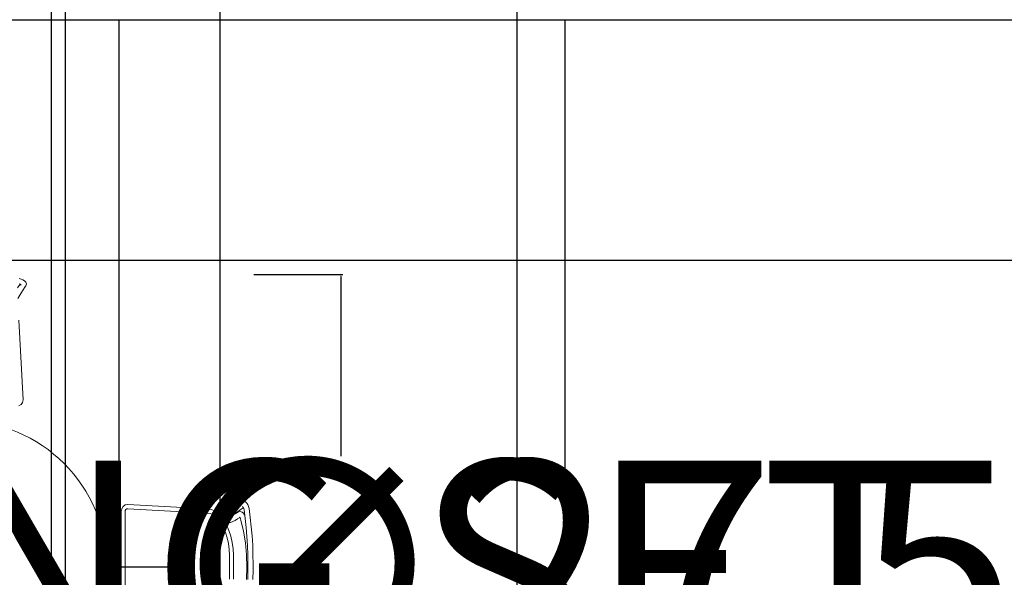
# Model space of a CAD drawing. Units: inches. Extents: x 305 to 776, y 38 to 479.
# Tile 11 of 14: x 419 to 511, y 280 to 332. Entities that reach past the tile are written whole.
import ezdxf

# ---------------------------------------------------------------- set-up
doc = ezdxf.new("R2010")
doc.units = ezdxf.units.IN
doc.header["$MEASUREMENT"] = 0
doc.layers.add('A-ANNO-DIMS', color=2, linetype='Continuous', lineweight=18)
doc.layers.add('A-FURN', color=8, linetype='Continuous', lineweight=18)
doc.styles.get("Standard").update_dxf_attribs({"font": 'arial.ttf'})
doc.dimstyles.get("Standard").update_dxf_attribs({"dimtxt": 20, "dimasz": 0.18, "dimexe": 0.18, "dimexo": 0.0625, "dimgap": 0.09, "dimtad": 0, "dimtih": 1, "dimtoh": 1, "dimdec": 4, "dimzin": 0, "dimdsep": 46, "dimtxsty": 'Standard', "dimcen": 0.09, "dimadec": 0, "dimazin": 0, "dimtfac": 1, "dimtdec": 4, "dimtofl": 0, "dimtmove": 0, "dimatfit": 3, "dimfxl": 1, "dimtolj": 1, "dimtzin": 0, "dimarcsym": 0})

# ---------------------------------------------------------------- blocks, each defined once
blk = doc.blocks.new('D')
for p, q in [((1089.75, 532.53), (1089.48, 532.6)), ((1089.75, 532.53), (1089.48, 532.6)), ((1089.62, 531.85), (1089.49, 531.9)), ((1089.97, 532.44), (1089.75, 532.53)), ((1089.97, 532.44), (1089.75, 532.53)), ((1090.18, 532.32), (1089.97, 532.44)), ((1090.18, 532.32), (1089.97, 532.44)), ((1090.35, 532.14), (1090.18, 532.32)), ((1090.35, 532.14), (1090.18, 532.32)), ((1090.39, 532.03), (1090.35, 532.14)), ((1090.35, 532.14), (1090.39, 532.03)), ((1090.43, 531.89), (1090.39, 532.03)), ((1090.43, 531.89), (1090.39, 532.03)), ((1090.4, 531.77), (1090.43, 531.89)), ((1090.43, 531.89), (1090.4, 531.77)), ((1089.27, 531.38), (1089.61, 531.85)), ((1089.58, 530.46), (1089.93, 531)), ((1089.58, 530.46), (1089.93, 531)), ((1089.69, 531.81), (1089.62, 531.85)), ((1089.78, 531.72), (1089.69, 531.81)), ((1089.93, 531), (1090.33, 531.61)), ((1089.93, 531), (1090.33, 531.61)), ((1090.33, 531.61), (1090.37, 531.66)), ((1090.37, 531.66), (1090.33, 531.61)), ((1090.37, 531.66), (1090.4, 531.77)), ((1090.37, 531.66), (1090.4, 531.77)), ((1089.31, 530.03), (1089.58, 530.46)), ((1089.31, 530.03), (1089.58, 530.46)), ((1090.02, 516.87), (1089.45, 527.19)), ((1090.02, 516.88), (1089.45, 527.19)), ((1089.95, 516.55), (1090.02, 516.88)), ((1089.95, 516.55), (1090.02, 516.87)), ((1089.44, 516.1), (1089.74, 516.28)), ((1089.44, 516.1), (1089.74, 516.28)), ((1089.74, 516.28), (1089.95, 516.55)), ((1089.74, 516.28), (1089.95, 516.55)), ((1102.72, 502.39), (1102.79, 502.75)), ((1102.72, 502.39), (1102.79, 502.75)), ((1102.79, 502.75), (1102.97, 503.06)), ((1102.79, 502.75), (1102.97, 503.06)), ((1102.97, 503.06), (1103.24, 503.26)), ((1102.97, 503.06), (1103.24, 503.26)), ((1103.24, 503.26), (1103.56, 503.33)), ((1103.24, 503.26), (1103.56, 503.33)), ((1103.33, 502.65), (1103.25, 502.53)), ((1103.43, 502.74), (1103.33, 502.65)), ((1103.56, 502.77), (1103.43, 502.74)), ((1103.56, 503.33), (1113.87, 502.77)), ((1103.56, 503.33), (1113.87, 502.77)), ((1113.85, 502.2), (1103.56, 502.77)), ((1113.87, 502.77), (1114.37, 502.68)), ((1113.87, 502.77), (1114.37, 502.68)), ((1114.37, 502.68), (1114.85, 502.5)), ((1114.37, 502.68), (1114.85, 502.5)), ((1116.01, 502.14), (1116.72, 502.62)), ((1116.01, 502.14), (1116.72, 502.62)), ((1116.72, 502.62), (1117.14, 502.89)), ((1116.72, 502.62), (1117.14, 502.89)), ((1117.14, 502.89), (1117.69, 503.24)), ((1117.14, 502.89), (1117.69, 503.24)), ((1117.56, 502.18), (1118.07, 502.58)), ((1117.69, 503.24), (1118.3, 503.64)), ((1117.69, 503.24), (1118.3, 503.64)), ((1118.07, 502.58), (1118.54, 502.93)), ((1118.3, 503.64), (1118.35, 503.68)), ((1118.35, 503.68), (1118.3, 503.64)), ((1118.35, 503.68), (1118.45, 503.71)), ((1118.35, 503.68), (1118.46, 503.71)), ((1118.41, 503.09), (1118.49, 503)), ((1118.45, 503.71), (1118.58, 503.74)), ((1118.58, 503.74), (1118.46, 503.71)), ((1118.49, 503), (1118.53, 502.93)), ((1118.53, 502.93), (1118.59, 502.8)), ((1118.58, 503.74), (1118.72, 503.7)), ((1118.58, 503.74), (1118.72, 503.7)), ((1118.59, 502.8), (1118.63, 502.63)), ((1118.63, 502.63), (1118.77, 501.51)), ((1118.72, 503.7), (1118.83, 503.66)), ((1118.83, 503.66), (1118.72, 503.7)), ((1118.83, 503.66), (1119.01, 503.49)), ((1118.83, 503.66), (1119.01, 503.49)), ((1119.01, 503.49), (1119.13, 503.29)), ((1119.01, 503.49), (1119.13, 503.29)), ((1119.13, 503.29), (1119.22, 503.06)), ((1119.13, 503.29), (1119.22, 503.06)), ((1119.22, 503.06), (1119.29, 502.79)), ((1119.22, 503.06), (1119.29, 502.79)), ((1119.29, 502.79), (1119.44, 501.61)), ((1119.29, 502.79), (1119.44, 501.61)), ((1102.72, 488.01), (1102.72, 502.39)), ((1102.72, 488.01), (1102.72, 502.39)), ((1103.25, 502.53), (1103.23, 502.39)), ((1103.23, 502.39), (1103.23, 488.01)), ((1114.27, 502.13), (1113.85, 502.2)), ((1114.68, 501.97), (1114.27, 502.13)), ((1115.05, 501.72), (1114.68, 501.97)), ((1114.85, 502.5), (1115.29, 502.22)), ((1114.85, 502.5), (1115.29, 502.22)), ((1115.37, 501.4), (1115.05, 501.72)), ((1115.29, 502.22), (1115.84, 501.82)), ((1115.29, 502.22), (1115.84, 501.82)), ((1115.63, 501.02), (1115.37, 501.4)), ((1115.84, 501.82), (1115.88, 501.74)), ((1116.37, 500.71), (1115.84, 501.82)), ((1115.88, 501.74), (1115.9, 501.76)), ((1115.89, 501.83), (1115.9, 501.9)), ((1115.9, 501.76), (1115.89, 501.83)), ((1115.9, 501.86), (1115.93, 502.01)), ((1115.9, 501.9), (1115.91, 501.96)), ((1115.91, 501.71), (1115.9, 501.86)), ((1115.91, 501.96), (1115.94, 502.03)), ((1115.98, 501.57), (1115.91, 501.71)), ((1115.93, 502.01), (1116.01, 502.14)), ((1115.94, 502.03), (1115.97, 502.09)), ((1115.97, 502.09), (1116.01, 502.14)), ((1116.08, 501.47), (1115.98, 501.57)), ((1116.21, 501.41), (1116.08, 501.47)), ((1116.35, 501.41), (1116.21, 501.41)), ((1116.48, 501.47), (1116.35, 501.41)), ((1116.66, 501.63), (1116.48, 501.47)), ((1116.53, 501.37), (1116.56, 501.49)), ((1116.54, 501.24), (1116.53, 501.37)), ((1116.56, 501.49), (1116.62, 501.59)), ((1116.62, 501.59), (1116.71, 501.67)), ((1116.88, 501.77), (1116.71, 501.67)), ((1116.88, 501.77), (1116.91, 501.79)), ((1116.91, 501.79), (1117.18, 501.93)), ((1117.18, 501.93), (1117.5, 502.11)), ((1117.41, 502.06), (1117.56, 502.18)), ((1117.47, 501.25), (1117.8, 501.44)), ((1117.5, 502.11), (1117.91, 502.35)), ((1117.8, 501.44), (1118.1, 501.61)), ((1117.91, 502.35), (1118.14, 502.39)), ((1118, 501.66), (1118.07, 501.64)), ((1118.07, 501.64), (1118.09, 501.63)), ((1118.09, 501.63), (1118.13, 501.57)), ((1118.13, 501.57), (1118.18, 501.45)), ((1118.26, 502.35), (1118.14, 502.39)), ((1118.18, 501.45), (1118.23, 501.29)), ((1118.23, 501.29), (1118.56, 499.86)), ((1118.26, 502.35), (1118.37, 502.32)), ((1118.37, 502.32), (1118.55, 502.17)), ((1118.55, 502.17), (1118.69, 501.98)), ((1118.69, 501.98), (1118.72, 501.92)), ((1118.77, 501.51), (1118.9, 500.35)), ((1119.44, 501.61), (1119.57, 500.43)), ((1119.44, 501.61), (1119.57, 500.43)), ((1115.96, 500.36), (1115.63, 501.02)), ((1116.23, 499.68), (1115.96, 500.36)), ((1116.37, 500.71), (1116.68, 499.96)), ((1116.58, 501.13), (1116.54, 501.24)), ((1116.66, 501.04), (1116.58, 501.13)), ((1116.76, 500.98), (1116.66, 501.04)), ((1116.87, 500.96), (1116.76, 500.98)), ((1116.87, 500.96), (1117.19, 501.11)), ((1117.19, 501.11), (1117.47, 501.25)), ((1118.9, 500.35), (1119, 499.17)), ((1119.57, 500.43), (1119.67, 499.23)), ((1119.57, 500.43), (1119.67, 499.23)), ((1116.45, 498.97), (1116.23, 499.68)), ((1116.61, 498.24), (1116.45, 498.97)), ((1116.68, 499.96), (1116.93, 499.19)), ((1116.93, 499.19), (1117.11, 498.39)), ((1118.56, 499.86), (1118.81, 498.35)), ((1119, 499.17), (1119.08, 497.98)), ((1119.67, 499.23), (1119.75, 498.02)), ((1119.67, 499.23), (1119.75, 498.02)), ((1116.71, 497.49), (1116.61, 498.24)), ((1116.75, 496.74), (1116.71, 497.49)), ((1117.11, 498.39), (1117.22, 497.57)), ((1117.22, 497.57), (1117.25, 496.74)), ((1118.81, 498.35), (1118.96, 496.79)), ((1119.08, 497.98), (1119.12, 496.78)), ((1119.75, 498.02), (1119.79, 496.8)), ((1119.75, 498.02), (1119.79, 496.8)), ((1116.75, 493.65), (1116.75, 496.74)), ((1117.25, 496.74), (1117.25, 493.65)), ((1118.96, 496.79), (1118.99, 495.2)), ((1119.12, 496.78), (1119.14, 495.57)), ((1119.79, 496.8), (1119.81, 495.58)), ((1119.79, 496.8), (1119.81, 495.58)), ((1118.96, 493.61), (1118.99, 495.2)), ((1119.14, 494.82), (1119.14, 495.57)), ((1119.81, 495.58), (1119.81, 494.82)), ((1119.81, 494.82), (1119.81, 495.58)), ((1119.12, 493.61), (1119.14, 494.82)), ((1119.81, 494.82), (1119.79, 493.59)), ((1119.79, 493.59), (1119.81, 494.82))]:
    blk.add_line(p, q)
blk.add_circle((1081.88, 495.2), 18.99)
blk = doc.blocks.new('*D19')
at = {"layer": 'A-ANNO-DIMS', "color": 0, "lineweight": -2, "transparency": 16777216}
for p, q in [((557.633, 250.82), (557.633, 245.977)), ((589.133, 250.82), (589.133, 245.977)), ((557.633, 246.157), (557.453, 246.157)), ((588.953, 246.157), (557.813, 246.157))]:
    blk.add_line(p, q, dxfattribs=at)
at = {"layer": 'A-ANNO-DIMS', "color": 0, "transparency": 16777216}
for points in [[(557.813, 246.187), (557.813, 246.127), (557.633, 246.157)], [(588.953, 246.187), (588.953, 246.127), (589.133, 246.157)]]:
    blk.add_solid(points, dxfattribs=at)
at = {"layer": 'Defpoints', "color": 0, "transparency": 16777216}
for p in [(557.633, 250.882), (589.133, 250.882), (557.633, 246.157)]:
    blk.add_point(p, dxfattribs=at)
at = {"layer": 'A-ANNO-DIMS', "color": 0, "transparency": 16777216, "insert": (463.393, 246.157), "char_height": 20, "attachment_point": 5}
blk.add_mtext('\\A1;DOOR 32 TYP.', dxfattribs=at)
blk = doc.blocks.new('*D20')
at = {"layer": 'A-ANNO-DIMS', "color": 0, "lineweight": -2, "transparency": 16777216}
for p, q in [((557.57, 280.724), (552.728, 280.724)), ((552.908, 280.544), (552.908, 276.111)), ((552.908, 251.062), (552.908, 255.495)), ((557.57, 250.882), (552.728, 250.882))]:
    blk.add_line(p, q, dxfattribs=at)
at = {"layer": 'A-ANNO-DIMS', "color": 0, "transparency": 16777216}
for points in [[(552.878, 280.544), (552.938, 280.544), (552.908, 280.724)], [(552.878, 251.062), (552.938, 251.062), (552.908, 250.882)]]:
    blk.add_solid(points, dxfattribs=at)
at = {"layer": 'Defpoints', "color": 0, "transparency": 16777216}
for p in [(552.908, 280.724), (557.633, 280.724), (557.633, 250.882)]:
    blk.add_point(p, dxfattribs=at)
at = {"layer": 'A-ANNO-DIMS', "color": 0, "transparency": 16777216, "insert": (552.908, 265.803), "char_height": 20, "attachment_point": 5}
blk.add_mtext('\\A1;30 TYP.', dxfattribs=at)
blk = doc.blocks.new('*D33')
at = {"layer": 'A-ANNO-DIMS', "color": 0, "lineweight": -2, "transparency": 16777216}
for p, q in [((440.927, 307.949), (449.29, 307.949)), ((449.11, 307.769), (449.11, 290.896)), ((449.11, 253.161), (449.11, 270.034)), ((440.927, 252.981), (449.29, 252.981))]:
    blk.add_line(p, q, dxfattribs=at)
at = {"layer": 'A-ANNO-DIMS', "color": 0, "transparency": 16777216}
for points in [[(449.08, 307.769), (449.14, 307.769), (449.11, 307.949)], [(449.08, 253.161), (449.14, 253.161), (449.11, 252.981)]]:
    blk.add_solid(points, dxfattribs=at)
at = {"layer": 'Defpoints', "color": 0, "transparency": 16777216}
for p in [(440.864, 307.949), (449.11, 307.949), (440.864, 252.981)]:
    blk.add_point(p, dxfattribs=at)
at = {"layer": 'A-ANNO-DIMS', "color": 0, "transparency": 16777216, "insert": (449.11, 280.465), "char_height": 20, "attachment_point": 5}
blk.add_mtext('\\A1;DINING SET 55', dxfattribs=at)
blk = doc.blocks.new('*D47')
at = {"layer": 'A-ANNO-DIMS', "color": 0, "lineweight": -2, "transparency": 16777216}
for p, q in [((465.633, 331.82), (465.633, 51.201)), ((470.133, 331.82), (470.133, 51.201)), ((465.813, 51.381), (469.953, 51.381)), ((470.133, 51.381), (470.313, 51.381))]:
    blk.add_line(p, q, dxfattribs=at)
at = {"layer": 'A-ANNO-DIMS', "color": 0, "transparency": 16777216}
for points in [[(465.813, 51.411), (465.813, 51.351), (465.633, 51.381)], [(469.953, 51.411), (469.953, 51.351), (470.133, 51.381)]]:
    blk.add_solid(points, dxfattribs=at)
at = {"layer": 'Defpoints', "color": 0, "transparency": 16777216}
for p in [(465.633, 331.882), (470.133, 331.882), (470.133, 51.381)]:
    blk.add_point(p, dxfattribs=at)
at = {"layer": 'A-ANNO-DIMS', "color": 0, "transparency": 16777216, "insert": (489.086, 51.381), "char_height": 20, "attachment_point": 5}
blk.add_mtext('\\A1;4.5', dxfattribs=at)
blk = doc.blocks.new('*D49')
at = {"layer": 'A-ANNO-DIMS', "color": 0, "lineweight": -2, "transparency": 16777216}
for p, q in [((399.695, 331.882), (648.814, 331.882)), ((648.634, 331.702), (648.634, 330.883)), ((648.634, 309.462), (648.634, 310.281)), ((399.695, 309.282), (648.814, 309.282))]:
    blk.add_line(p, q, dxfattribs=at)
at = {"layer": 'A-ANNO-DIMS', "color": 0, "transparency": 16777216}
for points in [[(648.604, 331.702), (648.664, 331.702), (648.634, 331.882)], [(648.604, 309.462), (648.664, 309.462), (648.634, 309.282)]]:
    blk.add_solid(points, dxfattribs=at)
at = {"layer": 'Defpoints', "color": 0, "transparency": 16777216}
for p in [(399.633, 331.882), (648.634, 331.882), (399.633, 309.282)]:
    blk.add_point(p, dxfattribs=at)
at = {"layer": 'A-ANNO-DIMS', "color": 0, "transparency": 16777216, "insert": (648.634, 320.582), "char_height": 20, "attachment_point": 5}
blk.add_mtext('\\A1;22.6', dxfattribs=at)
blk = doc.blocks.new('*D60')
at = {"layer": 'A-ANNO-DIMS', "color": 0, "lineweight": -2, "transparency": 16777216}
for p, q in [((428.263, 331.82), (428.263, 51.201)), ((465.633, 331.82), (465.633, 51.201)), ((428.443, 51.381), (465.453, 51.381)), ((465.633, 51.381), (465.813, 51.381))]:
    blk.add_line(p, q, dxfattribs=at)
at = {"layer": 'A-ANNO-DIMS', "color": 0, "transparency": 16777216}
for points in [[(428.443, 51.411), (428.443, 51.351), (428.263, 51.381)], [(465.453, 51.411), (465.453, 51.351), (465.633, 51.381)]]:
    blk.add_solid(points, dxfattribs=at)
at = {"layer": 'Defpoints', "color": 0, "transparency": 16777216}
for p in [(428.263, 331.882), (465.633, 331.882), (465.633, 51.381)]:
    blk.add_point(p, dxfattribs=at)
at = {"layer": 'A-ANNO-DIMS', "color": 0, "transparency": 16777216, "insert": (499.641, 51.381), "char_height": 20, "attachment_point": 5}
blk.add_mtext('\\A1;37.37', dxfattribs=at)
blk = doc.blocks.new('*D61')
at = {"layer": 'A-ANNO-DIMS', "color": 0, "lineweight": -2, "transparency": 16777216}
for p, q in [((437.73, 398.686), (437.73, 51.201)), ((465.633, 398.686), (465.633, 51.201)), ((437.91, 51.381), (465.453, 51.381)), ((465.633, 51.381), (465.813, 51.381))]:
    blk.add_line(p, q, dxfattribs=at)
at = {"layer": 'A-ANNO-DIMS', "color": 0, "transparency": 16777216}
for points in [[(437.91, 51.411), (437.91, 51.351), (437.73, 51.381)], [(465.453, 51.411), (465.453, 51.351), (465.633, 51.381)]]:
    blk.add_solid(points, dxfattribs=at)
at = {"layer": 'Defpoints', "color": 0, "transparency": 16777216}
for p in [(437.73, 398.749), (465.633, 398.749), (465.633, 51.381)]:
    blk.add_point(p, dxfattribs=at)
at = {"layer": 'A-ANNO-DIMS', "color": 0, "transparency": 16777216, "insert": (492.069, 51.381), "char_height": 20, "attachment_point": 5}
blk.add_mtext('\\A1;27.9', dxfattribs=at)
blk = doc.blocks.new('*D62')
at = {"layer": 'A-ANNO-DIMS', "color": 0, "lineweight": -2, "transparency": 16777216}
for p, q in [((399.633, 336.32), (399.633, 51.201)), ((423.233, 336.32), (423.233, 51.201)), ((399.813, 51.381), (423.053, 51.381)), ((423.233, 51.381), (423.413, 51.381))]:
    blk.add_line(p, q, dxfattribs=at)
at = {"layer": 'A-ANNO-DIMS', "color": 0, "transparency": 16777216}
for points in [[(399.813, 51.411), (399.813, 51.351), (399.633, 51.381)], [(423.053, 51.411), (423.053, 51.351), (423.233, 51.381)]]:
    blk.add_solid(points, dxfattribs=at)
at = {"layer": 'Defpoints', "color": 0, "transparency": 16777216}
for p in [(399.633, 336.382), (423.233, 336.382), (423.233, 51.381)]:
    blk.add_point(p, dxfattribs=at)
at = {"layer": 'A-ANNO-DIMS', "color": 0, "transparency": 16777216, "insert": (449.642, 51.381), "char_height": 20, "attachment_point": 5}
blk.add_mtext('\\A1;23.6', dxfattribs=at)
blk = doc.blocks.new('*D65')
at = {"layer": 'A-ANNO-DIMS', "color": 0, "lineweight": -2, "transparency": 16777216}
for p, q in [((399.633, 351.219), (399.633, 51.201)), ((421.89, 351.219), (421.89, 51.201)), ((399.813, 51.381), (421.71, 51.381)), ((421.89, 51.381), (422.07, 51.381))]:
    blk.add_line(p, q, dxfattribs=at)
at = {"layer": 'A-ANNO-DIMS', "color": 0, "transparency": 16777216}
for points in [[(399.813, 51.411), (399.813, 51.351), (399.633, 51.381)], [(421.71, 51.411), (421.71, 51.351), (421.89, 51.381)]]:
    blk.add_solid(points, dxfattribs=at)
at = {"layer": 'Defpoints', "color": 0, "transparency": 16777216}
for p in [(399.633, 351.281), (421.89, 351.281), (421.89, 51.381)]:
    blk.add_point(p, dxfattribs=at)
at = {"layer": 'A-ANNO-DIMS', "color": 0, "transparency": 16777216, "insert": (463.844, 51.381), "char_height": 20, "attachment_point": 5}
blk.add_mtext('\\A1;22.257', dxfattribs=at)
blk = doc.blocks.new('*D75')
at = {"layer": 'A-ANNO-DIMS', "color": 0, "lineweight": -2, "transparency": 16777216}
for p, q in [((413.291, 280.465), (413.471, 280.465)), ((413.381, 280.375), (413.381, 280.555)), ((435.396, 280.465), (427.32, 280.465))]:
    blk.add_line(p, q, dxfattribs=at)
at = {"layer": 'A-ANNO-DIMS', "color": 0, "transparency": 16777216}
blk.add_solid([(427.32, 280.495), (427.32, 280.435), (427.14, 280.465)], dxfattribs=at)
at = {"layer": 'Defpoints', "color": 0, "transparency": 16777216}
for p in [(399.621, 280.466), (427.14, 280.465)]:
    blk.add_point(p, dxfattribs=at)
at = {"layer": 'A-ANNO-DIMS', "color": 0, "transparency": 16777216, "insert": (480.009, 280.465), "char_height": 20, "attachment_point": 5}
blk.add_mtext('\\A1;∅27.52', dxfattribs=at)

msp = doc.modelspace()

# ---------------------------------------------------------------- block references
at = {"layer": 'A-FURN', "xscale": 0.724692399516523, "yscale": 0.724692399516523, "zscale": 0.724692399516523}
msp.add_blockref('D', (-370.653, -78.4001), dxfattribs=at)

# ---------------------------------------------------------------- dimensions: what is measured, and where the dimension line sits
at = {"layer": 'A-ANNO-DIMS'}
for base, p1, p2, override, picture, middle in [((465.6329, 51.3805), (437.7303, 398.7487), (465.6329, 398.7487), {"dimdec": 1, "dimlfac": 1, "dimrnd": 0, "dimzin": 0, "dimdsep": 46, "dimlunit": 2}, '*D61', (492.0693, 51.3805)), ((421.8895, 51.3805), (399.6329, 351.2815), (421.8895, 351.2815), {"dimdec": 3, "dimlfac": 1, "dimrnd": 0, "dimzin": 0, "dimdsep": 46, "dimlunit": 2}, '*D65', (463.8444, 51.3805)), ((423.2329, 51.3805), (399.6329, 336.382), (423.2329, 336.382), {"dimdec": 1, "dimlfac": 1, "dimrnd": 0, "dimzin": 0, "dimdsep": 46, "dimlunit": 2}, '*D62', (449.6421, 51.3805)), ((465.6329, 51.3805), (428.2629, 331.882), (465.6329, 331.882), {"dimdec": 2, "dimlfac": 1, "dimrnd": 0, "dimzin": 0, "dimdsep": 46, "dimlunit": 2}, '*D60', (499.641, 51.3805)), ((470.1329, 51.3805), (465.6329, 331.882), (470.1329, 331.882), {"dimdec": 1, "dimlfac": 1, "dimrnd": 0, "dimzin": 0, "dimdsep": 46, "dimlunit": 2}, '*D47', (489.0864, 51.3805))]:
    dim = msp.add_linear_dim(base=base, p1=p1, p2=p2, dimstyle='Standard', override=override, dxfattribs=at)
    dim.commit()
    dim.dimension.update_dxf_attribs({"geometry": picture, "text_midpoint": middle})
dim = msp.add_linear_dim(base=(648.6344, 331.882), p1=(399.6329, 309.2819), p2=(399.6329, 331.882), angle=90, dimstyle='Standard', override={"dimdec": 1, "dimlfac": 1, "dimrnd": 0, "dimzin": 0, "dimdsep": 46, "dimlunit": 2}, dxfattribs=at)
dim.commit()
dim.dimension.update_dxf_attribs({"geometry": '*D49', "text_midpoint": (648.6344, 320.582)})
for base, p1, p2, angle, text, picture, middle in [((449.1096, 307.9493), (440.8644, 252.9815), (440.8644, 307.9493), 90, 'DINING SET <>', '*D33', (449.1096, 280.4654)), ((552.9079, 280.7241), (557.6329, 250.882), (557.6329, 280.7241), 90, '<> TYP.', '*D20', (552.9079, 265.8031)), ((557.6329062952, 246.15704135), (589.1329062952, 250.88204135), (557.6329062952, 250.88204135), 180, 'DOOR <> TYP.', '*D19', (463.3929199378, 246.15704135))]:
    dim = msp.add_linear_dim(base=base, p1=p1, p2=p2, angle=angle, text=text, dimstyle='Standard', override={"dimdec": 0, "dimlfac": 1, "dimrnd": 0, "dimzin": 0, "dimdsep": 46, "dimlunit": 2}, dxfattribs=at)
    dim.commit()
    dim.dimension.update_dxf_attribs({"geometry": picture, "text_midpoint": middle})
dim = msp.add_diameter_dim_2p(p1=(399.6205, 280.4658), p2=(427.1405, 280.465), dimstyle='Standard', override={"dimdec": 2, "dimlfac": 1, "dimrnd": 0, "dimzin": 0, "dimdsep": 46, "dimlunit": 2}, dxfattribs=at)
dim.commit()
dim.dimension.update_dxf_attribs({"geometry": '*D75', "text_midpoint": (435.3965, 280.4648), "dimtype": 163})

doc.saveas('drawing.dxf')
